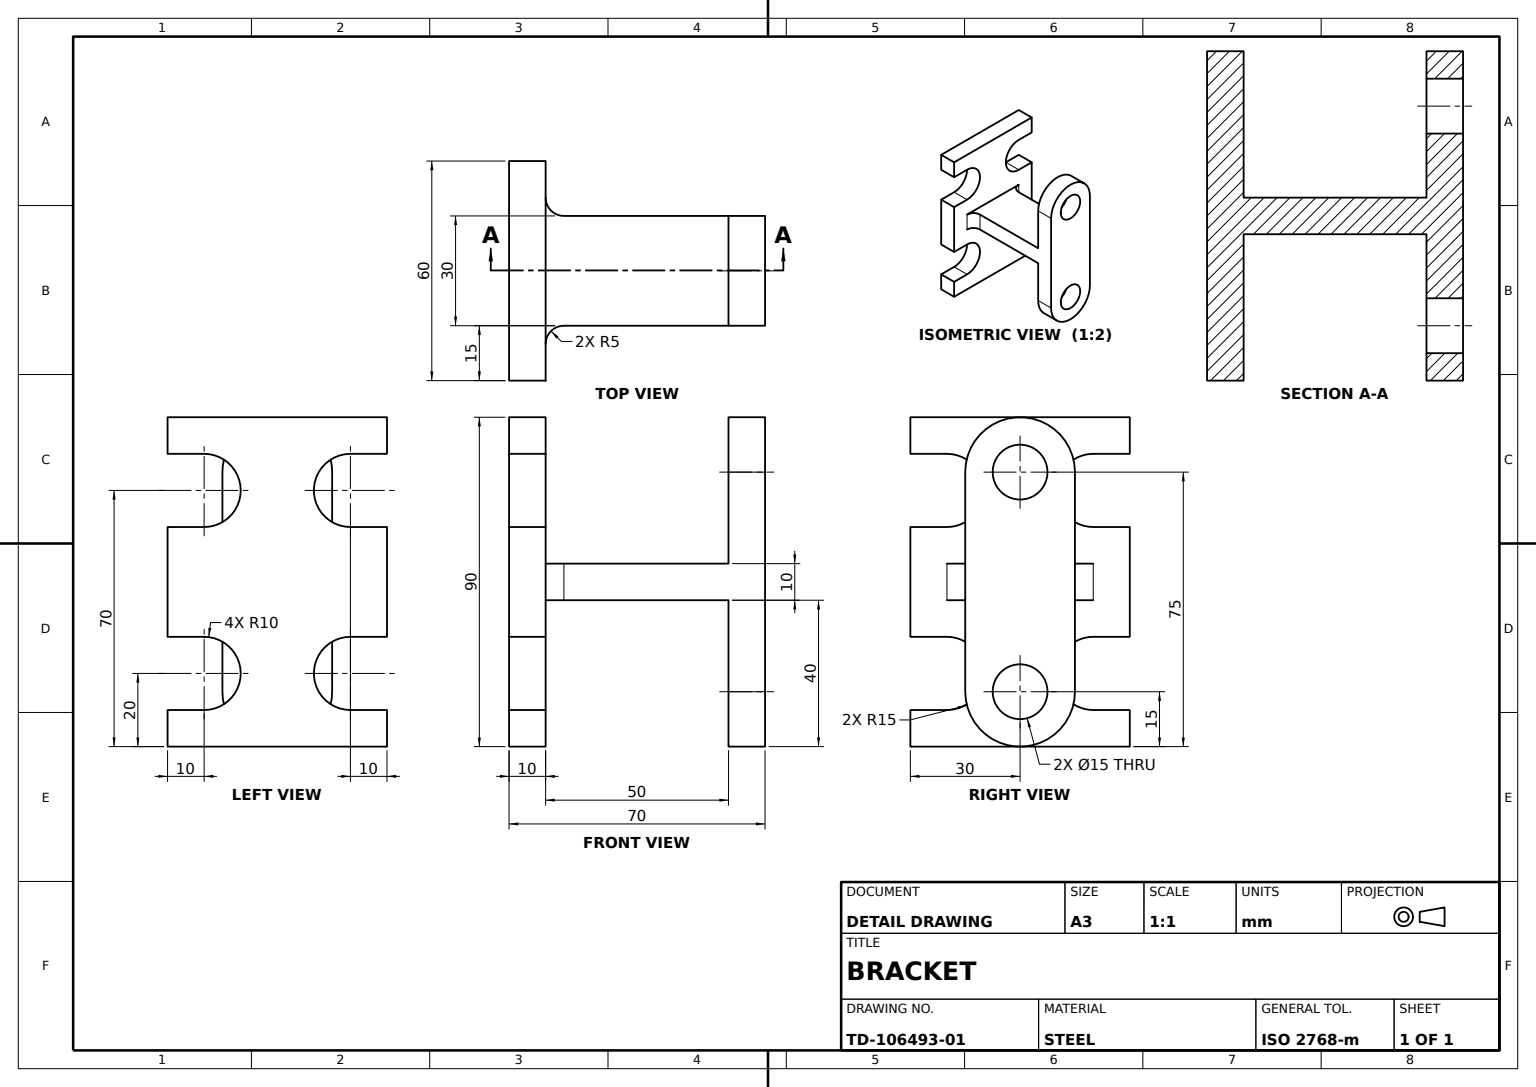
SolidWorks part; units mm, degrees
material "Plain Carbon Steel"
ref_plane "Front Plane" through (0, 0, 0) normal (0, 0, 1) x (1, 0, 0)
ref_plane "Top Plane" through (0, 0, 0) normal (0, 1, 0) x (1, 0, 0)
ref_plane "Right Plane" through (0, 0, 0) normal (1, 0, 0) x (0, 0, -1)
sketch "H Profile Sketch" plane through (0, 0, 0) normal (0, 0, 1) x (1, 0, 0)
  line L0 (0, 0) -> (0, 45)
  line L1 (0, 0) -> (0, -45)
  line L2 (0, -45) -> (10, -45)
  line L3 (10, -45) -> (10, -5)
  line L4 (10, 45) -> (0, 45)
  line L5 (10, 5) -> (10, 45)
  line L6 (60, 45) -> (60, -45)
  line L7 (60, -45) -> (50, -45)
  line L8 (50, -45) -> (50, -5)
  line L9 (50, 45) -> (60, 45)
  line L11 (10, 5) -> (50, 5)
  line L13 (50, -5) -> (10, -5)
  line L15 (50, 5) -> (50, 45)
  dimension "D1" = 10
  dimension "D2" = 50
  dimension "D3" = 45
extrude "H Body Extrude 60" add sketch "H Profile Sketch" along normal blind 60
sketch "Relief Cut Sketch" plane through (0, 0, 0) normal (-1, 0, 0) x (0, 0, 1)
  line L0 (0, 45) -> (0, 35)
  line L1 (0, 45) -> (0, -45) construction
  line L2 (0, 35) -> (10, 35)
  line L3 (0, 35) -> (0, 15)
  line L4 (10, 15) -> (0, 15)
  line L5 (0, 15) -> (0, -15)
  line L6 (0, -15) -> (10, -15)
  line L7 (0, -15) -> (0, -35)
  line L8 (10, -35) -> (0, -35)
  line L9 (0, -35) -> (0, -45)
  line L12 (60, -35) -> (60, -45)
  line L13 (50, -35) -> (60, -35)
  line L14 (60, -15) -> (50, -15)
  line L15 (60, 15) -> (60, -15)
  line L16 (50, 15) -> (60, 15)
  line L17 (60, 35) -> (50, 35)
  line L18 (60, 45) -> (60, 35)
  line L19 (0, 45) -> (60, 45)
  line L20 (0, -45) -> (60, -45)
  line L21 (60, 35) -> (60, 15)
  line L22 (60, -15) -> (60, -35)
  arc A0 (10, 15) -> (10, 35) centre (10, 25) ccw
  arc A1 (10, -15) -> (10, -35) centre (10, -25) cw
  arc A2 (50, -15) -> (50, -35) centre (50, -25) ccw
  arc A3 (50, 15) -> (50, 35) centre (50, 25) cw
  line M3 (0, 45) -> (0, -45)
  line M5 (60, -45) -> (60, 45)
  dimension "D1" = 10
  dimension "D2" = 50
extrude "Relief Cut 10" cut sketch "Relief Cut Sketch" against normal blind 10 contours L4 A0 L2 M3 | A3 L16 L17 M5 | A1 L6 L8 M3 | L14 A2 L13 M5
sketch "Connector Arm Sketch" plane through (60, 0, 0) normal (1, 0, 0) x (0, 0, -1)
  line L0 (-30, 45) -> (-30, -45) construction
  line L3 (0, -45) -> (0, 45) construction
  line L4 (-60, 45) -> (0, 45) construction
  line L5 (-30, 30) -> (-30, -30) construction
  line L7 (-15, 30) -> (-15, -30)
  line L8 (-45, 30) -> (-45, -30)
  arc A0 (-15, 30) -> (-45, 30) centre (-30, 30) ccw
  arc A1 (-45, -30) -> (-15, -30) centre (-30, -30) ccw
  circle A2 centre (-30, 30) radius 7.5
  circle A3 centre (-30, -30) radius 7.5
  point P13 (-30, 0)
  dimension "D1" = 15
  dimension "D3" = 15
  dimension "D2" = 60
  dimension "D4" = 30
  dimension "D5" = 15
extrude "Connector Arm Boss" add sketch "Connector Arm Sketch" against normal blind 10
sketch "Notch Cut A Sketch" plane through (50, 0, 0) normal (-1, 0, 0) x (0, 0, 1)
  line L0 (0, 45) -> (0, 5)
  line L1 (0, 45) -> (0, 5) construction
  line L2 (0, 5) -> (60, 5)
  line L3 (60, 5) -> (60, 45)
  line L4 (60, 45) -> (0, 45)
extrude "Notch Cut A" cut sketch "Notch Cut A Sketch" against normal blind 10
sketch "Notch Cut B Sketch" plane through (50, 0, 0) normal (-1, 0, 0) x (0, 0, 1)
  line L0 (0, -5) -> (60, -5)
  line L1 (60, -5) -> (60, -45)
  line L2 (60, -45) -> (0, -45)
  line L3 (0, -45) -> (0, -5)
extrude "Notch Cut B" cut sketch "Notch Cut B Sketch" against normal blind 10
sketch "Link Plate Sketch" plane through (60, 0, 0) normal (1, 0, 0) x (0, 0, -1)
  line L0 (-30, 5) -> (-30, 30) construction
  line L1 (-30, 30) -> (-30, -30) construction
  line L2 (-60, 5) -> (0, 5) construction
  line L3 (-60, -5) -> (0, -5) construction
  line L4 (-15, 30) -> (-15, -30)
  line L5 (-45, 30) -> (-45, -30)
  arc A0 (-15, 30) -> (-45, 30) centre (-30, 30) ccw
  arc A1 (-45, -30) -> (-15, -30) centre (-30, -30) ccw
  circle A2 centre (-30, 30) radius 7.5
  circle A3 centre (-30, -30) radius 7.5
  point P7 (-30, 0)
  dimension "D1" = 15
  dimension "D3" = 15
  dimension "D2" = 60
  dimension "D4" = 5
extrude "Link Plate Boss" add sketch "Link Plate Sketch" along normal blind 10
sketch "Link Plate Holes Sketch" plane through (0, 5, 0) normal (0, 1, 0) x (1, 0, 0)
  line L0 (60, -15) -> (10, -15)
  line L1 (10, -60) -> (10, 0) construction
  line L2 (10, -15) -> (10, 0)
  line L3 (10, 0) -> (60, 0)
  line L4 (60, 0) -> (60, -15)
  line L5 (60, -45) -> (10, -45)
  line L6 (10, -60) -> (10, 0) construction
  line L7 (10, -45) -> (10, -60)
  line L8 (10, -60) -> (60, -60)
  line L9 (60, -45) -> (60, -60) construction
  line L10 (60, -60) -> (10, -60) construction
  line L11 (60, -60) -> (60, -45)
extrude "Link Plate Holes" cut sketch "Link Plate Holes Sketch" against normal through all
fillet "Edge Fillets R5" radius 5 2 edges at (10, 0, 15) (10, 0, 45)
